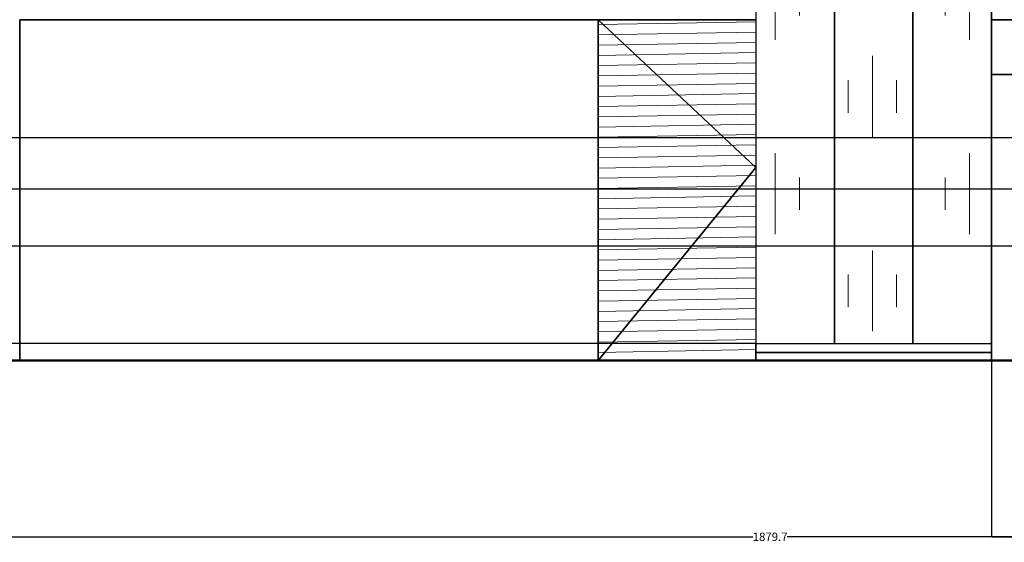
# Model space of a CAD drawing. Units: inches. Extents: x -1308 to 780, y 304 to 1023.
# Tile 3 of 7: x -667 to -138, y 304 to 585. Entities that reach past the tile are written whole.
import ezdxf

# ---------------------------------------------------------------- set-up
doc = ezdxf.new("R2010")
doc.units = ezdxf.units.IN
doc.header["$MEASUREMENT"] = 0
for name, color, linetype, lineweight in [('A-ANNO-DIMS', 2, 'Continuous', 18), ('A-ELEV', 7, 'Continuous', 35), ('A-ELEV-GRND', 7, 'Continuous', 50), ('A-ELEV-PATT', 8, 'Continuous', 13), ('A-GLAZ', 4, 'Continuous', 25)]:
    doc.layers.add(name, color=color, linetype=linetype, lineweight=lineweight)
doc.styles.get("Standard").update_dxf_attribs({"font": 'arial.ttf'})
doc.dimstyles.get("Standard").update_dxf_attribs({"dimtxt": 4.5, "dimasz": 0.18, "dimexe": 0.18, "dimexo": 0.0625, "dimgap": 0.09, "dimtad": 0, "dimtih": 1, "dimtoh": 1, "dimdec": 4, "dimzin": 0, "dimdsep": 46, "dimlunit": 4, "dimtxsty": 'Standard', "dimcen": 0.09, "dimadec": 0, "dimazin": 0, "dimtfac": 1, "dimtdec": 4, "dimtofl": 0, "dimtmove": 0, "dimatfit": 3, "dimfxl": 1, "dimtolj": 1, "dimtzin": 0, "dimarcsym": 0})

# ---------------------------------------------------------------- blocks, each defined once
blk = doc.blocks.new('*D1')
at = {"layer": 'A-ANNO-DIMS', "color": 0, "lineweight": -2, "transparency": 16777216}
for p, q in [((-1203.52, 401.95), (-1203.52, 307.09)), ((676.16, 401.95), (676.16, 307.09)), ((-1203.34, 307.27), (-272.9, 307.27)), ((675.98, 307.27), (-254.46, 307.27))]:
    blk.add_line(p, q, dxfattribs=at)
at = {"layer": 'A-ANNO-DIMS', "color": 0, "transparency": 16777216}
for points in [[(-1203.34, 307.3), (-1203.34, 307.24), (-1203.52, 307.27)], [(675.98, 307.3), (675.98, 307.24), (676.16, 307.27)]]:
    blk.add_solid(points, dxfattribs=at)
at = {"layer": 'Defpoints', "color": 0, "transparency": 16777216}
for p in [(-1203.52, 402.02), (676.16, 402.02), (676.16, 307.27)]:
    blk.add_point(p, dxfattribs=at)
at = {"layer": 'A-ANNO-DIMS', "color": 0, "transparency": 16777216, "insert": (-263.68, 307.27), "char_height": 4.5, "attachment_point": 5}
blk.add_mtext('\\A1;1879.7', dxfattribs=at)
blk = doc.blocks.new('*D9')
at = {"layer": 'A-ANNO-DIMS', "color": 0, "lineweight": -2, "transparency": 16777216}
for p, q in [((-144.73, 555.46), (-144.73, 307.09)), ((-129.95, 555.46), (-129.95, 307.09)), ((-144.55, 307.27), (-130.13, 307.27)), ((-129.95, 307.27), (-129.77, 307.27))]:
    blk.add_line(p, q, dxfattribs=at)
at = {"layer": 'A-ANNO-DIMS', "color": 0, "transparency": 16777216}
for points in [[(-144.55, 307.3), (-144.55, 307.24), (-144.73, 307.27)], [(-130.13, 307.3), (-130.13, 307.24), (-129.95, 307.27)]]:
    blk.add_solid(points, dxfattribs=at)
at = {"layer": 'Defpoints', "color": 0, "transparency": 16777216}
for p in [(-144.73, 555.52), (-129.95, 555.52), (-129.95, 307.27)]:
    blk.add_point(p, dxfattribs=at)
at = {"layer": 'A-ANNO-DIMS', "color": 0, "transparency": 16777216, "insert": (-120.55, 307.27), "char_height": 4.5, "attachment_point": 5}
blk.add_mtext('\\A1;14.787', dxfattribs=at)
blk = doc.blocks.new('*D45')
at = {"layer": 'A-ANNO-DIMS', "color": 0, "lineweight": -2, "transparency": 16777216}
for p, q in [((-25.86, 614.44), (-25.86, 307.09)), ((-144.73, 584.98), (-144.73, 307.09)), ((-144.55, 307.27), (-94.52, 307.27)), ((-26.04, 307.27), (-76.07, 307.27))]:
    blk.add_line(p, q, dxfattribs=at)
at = {"layer": 'A-ANNO-DIMS', "color": 0, "transparency": 16777216}
for points in [[(-144.55, 307.3), (-144.55, 307.24), (-144.73, 307.27)], [(-26.04, 307.3), (-26.04, 307.24), (-25.86, 307.27)]]:
    blk.add_solid(points, dxfattribs=at)
at = {"layer": 'Defpoints', "color": 0, "transparency": 16777216}
for p in [(-25.86, 614.51), (-144.73, 585.04), (-25.86, 307.27)]:
    blk.add_point(p, dxfattribs=at)
at = {"layer": 'A-ANNO-DIMS', "color": 0, "transparency": 16777216, "insert": (-85.3, 307.27), "char_height": 4.5, "attachment_point": 5}
blk.add_mtext('\\A1;118.88', dxfattribs=at)
blk = doc.blocks.new('*D57')
at = {"layer": 'A-ANNO-DIMS', "color": 0, "lineweight": -2, "transparency": 16777216}
for p, q in [((-628.74, 924.84), (-1298.45, 924.84)), ((-1298.27, 924.66), (-1298.27, 665.82)), ((-1298.27, 402.2), (-1298.27, 661.04)), ((-1203.58, 402.02), (-1298.45, 402.02))]:
    blk.add_line(p, q, dxfattribs=at)
at = {"layer": 'A-ANNO-DIMS', "color": 0, "transparency": 16777216}
for points in [[(-1298.3, 924.66), (-1298.24, 924.66), (-1298.27, 924.84)], [(-1298.3, 402.2), (-1298.24, 402.2), (-1298.27, 402.02)]]:
    blk.add_solid(points, dxfattribs=at)
at = {"layer": 'Defpoints', "color": 0, "transparency": 16777216}
for p in [(-1298.27, 924.84), (-628.68, 924.84), (-1203.52, 402.02)]:
    blk.add_point(p, dxfattribs=at)
at = {"layer": 'A-ANNO-DIMS', "color": 0, "transparency": 16777216, "insert": (-1298.27, 663.43), "char_height": 4.5, "attachment_point": 5}
blk.add_mtext('\\A1;522.8', dxfattribs=at)
blk = doc.blocks.new('*D58')
at = {"layer": 'A-ANNO-DIMS', "color": 0, "lineweight": -2, "transparency": 16777216}
for p, q in [((-1187.44, 521.84), (771.09, 521.84)), ((770.91, 521.66), (770.91, 464.32)), ((770.91, 402.2), (770.91, 459.54)), ((-1187.44, 402.02), (771.09, 402.02))]:
    blk.add_line(p, q, dxfattribs=at)
at = {"layer": 'A-ANNO-DIMS', "color": 0, "transparency": 16777216}
for points in [[(770.88, 521.66), (770.94, 521.66), (770.91, 521.84)], [(770.88, 402.2), (770.94, 402.2), (770.91, 402.02)]]:
    blk.add_solid(points, dxfattribs=at)
at = {"layer": 'Defpoints', "color": 0, "transparency": 16777216}
for p in [(-1187.5, 521.84), (770.91, 521.84), (-1187.5, 402.02)]:
    blk.add_point(p, dxfattribs=at)
at = {"layer": 'A-ANNO-DIMS', "color": 0, "transparency": 16777216, "insert": (770.91, 461.93), "char_height": 4.5, "attachment_point": 5}
blk.add_mtext('\\A1;119.83', dxfattribs=at)
blk = doc.blocks.new('*D63')
at = {"layer": 'A-ANNO-DIMS', "color": 0, "lineweight": -2, "transparency": 16777216}
for p, q in [((-843.54, 629.44), (771.09, 629.44)), ((770.91, 629.26), (770.91, 518.12)), ((770.91, 402.2), (770.91, 513.34)), ((-843.54, 402.02), (771.09, 402.02))]:
    blk.add_line(p, q, dxfattribs=at)
at = {"layer": 'A-ANNO-DIMS', "color": 0, "transparency": 16777216}
for points in [[(770.88, 629.26), (770.94, 629.26), (770.91, 629.44)], [(770.88, 402.2), (770.94, 402.2), (770.91, 402.02)]]:
    blk.add_solid(points, dxfattribs=at)
at = {"layer": 'Defpoints', "color": 0, "transparency": 16777216}
for p in [(-843.6, 629.44), (770.91, 629.44), (-843.6, 402.02)]:
    blk.add_point(p, dxfattribs=at)
at = {"layer": 'A-ANNO-DIMS', "color": 0, "transparency": 16777216, "insert": (770.91, 515.73), "char_height": 4.5, "attachment_point": 5}
blk.add_mtext('\\A1;227.43', dxfattribs=at)
blk = doc.blocks.new('*D67')
at = {"layer": 'A-ANNO-DIMS', "color": 0, "lineweight": -2, "transparency": 16777216}
for p, q in [((-271.41, 600.04), (-1298.45, 600.04)), ((-1298.27, 599.86), (-1298.27, 507.96)), ((-1298.27, 411.28), (-1298.27, 503.18)), ((-271.41, 411.1), (-1298.45, 411.1))]:
    blk.add_line(p, q, dxfattribs=at)
at = {"layer": 'A-ANNO-DIMS', "color": 0, "transparency": 16777216}
for points in [[(-1298.3, 599.86), (-1298.24, 599.86), (-1298.27, 600.04)], [(-1298.3, 411.28), (-1298.24, 411.28), (-1298.27, 411.1)]]:
    blk.add_solid(points, dxfattribs=at)
at = {"layer": 'Defpoints', "color": 0, "transparency": 16777216}
for p in [(-1298.27, 600.04), (-271.35, 600.04), (-271.35, 411.1)]:
    blk.add_point(p, dxfattribs=at)
at = {"layer": 'A-ANNO-DIMS', "color": 0, "transparency": 16777216, "insert": (-1298.27, 505.57), "char_height": 4.5, "attachment_point": 5}
blk.add_mtext('\\A1;188.94', dxfattribs=at)
blk = doc.blocks.new('*D79')
at = {"layer": 'A-ANNO-DIMS', "color": 0, "lineweight": -2, "transparency": 16777216}
for p, q in [((310.7, 463.43), (-1298.45, 463.43)), ((-1298.27, 463.25), (-1298.27, 435.11)), ((-1298.27, 402.2), (-1298.27, 430.34)), ((296.47, 402.02), (-1298.45, 402.02))]:
    blk.add_line(p, q, dxfattribs=at)
at = {"layer": 'A-ANNO-DIMS', "color": 0, "transparency": 16777216}
for points in [[(-1298.3, 463.25), (-1298.24, 463.25), (-1298.27, 463.43)], [(-1298.3, 402.2), (-1298.24, 402.2), (-1298.27, 402.02)]]:
    blk.add_solid(points, dxfattribs=at)
at = {"layer": 'Defpoints', "color": 0, "transparency": 16777216}
for p in [(-1298.27, 463.43), (310.77, 463.43), (296.53, 402.02)]:
    blk.add_point(p, dxfattribs=at)
at = {"layer": 'A-ANNO-DIMS', "color": 0, "transparency": 16777216, "insert": (-1298.27, 432.72), "char_height": 4.5, "attachment_point": 5}
blk.add_mtext('\\A1;61.42', dxfattribs=at)
blk = doc.blocks.new('*D80')
at = {"layer": 'A-ANNO-DIMS', "color": 0, "lineweight": -2, "transparency": 16777216}
for p, q in [((308.7, 494.07), (-1298.45, 494.07)), ((-1298.27, 493.89), (-1298.27, 481.14)), ((-1298.27, 463.61), (-1298.27, 476.36)), ((310.7, 463.43), (-1298.45, 463.43))]:
    blk.add_line(p, q, dxfattribs=at)
at = {"layer": 'A-ANNO-DIMS', "color": 0, "transparency": 16777216}
for points in [[(-1298.3, 493.89), (-1298.24, 493.89), (-1298.27, 494.07)], [(-1298.3, 463.61), (-1298.24, 463.61), (-1298.27, 463.43)]]:
    blk.add_solid(points, dxfattribs=at)
at = {"layer": 'Defpoints', "color": 0, "transparency": 16777216}
for p in [(-1298.27, 494.07), (308.77, 494.07), (310.77, 463.43)]:
    blk.add_point(p, dxfattribs=at)
at = {"layer": 'A-ANNO-DIMS', "color": 0, "transparency": 16777216, "insert": (-1298.27, 478.75), "char_height": 4.5, "attachment_point": 5}
blk.add_mtext('\\A1;30.64', dxfattribs=at)

msp = doc.modelspace()

# ---------------------------------------------------------------- hatches: boundary and pattern name
at = {"layer": 'A-ELEV-PATT'}
h = msp.add_hatch(dxfattribs=at)
h.set_pattern_fill('GOST_GLASS', color=256, scale=8.7, angle=45)
h.set_pattern_definition([(90, (0, 0), (52.2, 52.2), [43.5, -60.9]), (90, (13.05, 13.05), (52.2, 52.2), [17.4, -87]), (90, (-13.05, 13.05), (52.2, 52.2), [17.4, -87])])
h.paths.add_polyline_path([(-570.795, 854.0948), (-613.9558, 854.0948), (-613.9558, 755.0385), (-570.795, 755.0385)])
h.paths.add_polyline_path([(-499.4748, 854.0948), (-568.795, 854.0948), (-568.795, 755.0385), (-499.4748, 755.0385)])
h.paths.add_polyline_path([(-379.8352, 854.0948), (-497.4748, 854.0948), (-497.4748, 755.0385), (-379.8352, 755.0385)])
h.paths.add_polyline_path([(-292.4461, 854.0948), (-377.8352, 854.0948), (-377.8352, 755.0385), (-292.4461, 755.0385)])
h.paths.add_polyline_path([(4.0783, 875.1709), (-63.0069, 875.1709), (-63.0069, 753.0385), (4.0783, 753.0385)])
h.paths.add_polyline_path([(77.4055, 875.1709), (6.0783, 875.1709), (6.0783, 753.0385), (77.4055, 753.0385)])
h.paths.add_polyline_path([(150.9148, 814.1047), (79.4055, 814.1047), (79.4055, 753.0385), (150.9148, 753.0385)])
h.paths.add_polyline_path([(110.9181, 875.1709), (79.4055, 875.1709), (79.4055, 814.1047)])
h.paths.add_polyline_path([(150.9148, 875.1709), (110.9181, 875.1709), (149.6048, 816.1047), (150.9148, 816.1047)])
h.paths.add_polyline_path([(-227.6882, 875.1709), (-271.346, 875.1709), (-271.346, 753.0385), (-227.6882, 753.0385)])
h.paths.add_polyline_path([(-188.3907, 875.1709), (-227.6882, 875.1709), (-227.6882, 753.0385), (-188.3907, 753.0385)])
h.paths.add_polyline_path([(-144.7329, 875.1709), (-188.3907, 875.1709), (-188.3907, 753.0385), (-144.7329, 753.0385)])
h.paths.add_polyline_path([(-144.7329, 739.0259), (-188.3907, 739.0259), (-188.3907, 624.4429), (-144.7329, 624.4429)])
h.paths.add_polyline_path([(-188.3907, 739.0259), (-227.6882, 739.0259), (-227.6882, 624.4429), (-188.3907, 624.4429)])
h.paths.add_polyline_path([(-227.6882, 739.0259), (-271.346, 739.0259), (-271.346, 624.4429), (-227.6882, 624.4429)])
h.paths.add_polyline_path([(-229.1416, 600.0434), (-271.346, 600.0434), (-271.346, 411.1006), (-229.1416, 411.1006)])
h.paths.add_polyline_path([(-186.9373, 600.0434), (-229.1416, 600.0434), (-229.1416, 411.1006), (-186.9373, 411.1006)])
h.paths.add_polyline_path([(-144.7329, 600.0434), (-186.9373, 600.0434), (-186.9373, 411.1006), (-144.7329, 411.1006)])
h = msp.add_hatch(dxfattribs=at)
h.set_pattern_fill('ANSI31', color=256, scale=44, angle=136)
h.paths.add_polyline_path([(-271.346, 505.572), (-356.0562, 585.0385), (-356.0562, 402.0158)])
h.paths.add_polyline_path([(-271.346, 585.0385), (-356.0562, 585.0385), (-271.346, 505.572)], flags=17)
h.paths.add_polyline_path([(-271.346, 505.572), (-356.0562, 402.0158), (-271.346, 402.0158), (-271.346, 406.2371), (-271.346, 411.1006)], flags=17)

# ---------------------------------------------------------------- linework, layer by layer
at = {"layer": 'A-ELEV'}
for p, q in [((-144.7329, 753.0385), (-144.7329, 585.0385)), ((-666.946, 402.0158), (-666.946, 585.0385)), ((-666.946, 585.0385), (-557.1914, 585.0385)), ((-271.346, 585.0385), (-557.1914, 585.0385)), ((-356.0562, 585.0385), (-356.0562, 402.0158)), ((-356.0562, 585.0385), (-271.346, 505.572)), ((-144.7329, 555.5236), (-144.7329, 585.0385)), ((-144.7329, 585.0385), (526.9606, 585.0385)), ((50.6624, 555.5236), (-144.7329, 555.5236)), ((-144.7329, 555.5236), (-144.7329, 402.0158)), ((-271.346, 505.572), (-356.0562, 402.0158)), ((-271.346, 411.1006), (-271.346, 406.2371)), ((-271.346, 406.2371), (-144.7329, 406.2371)), ((-271.346, 406.2371), (-271.346, 402.0158))]:
    msp.add_line(p, q, dxfattribs=at)
at = {"layer": 'A-ELEV-GRND'}
for p, q in [((-608.7933, 402.0158), (-725.0987, 402.0158)), ((-144.7329, 402.0158), (-608.7933, 402.0158)), ((47.1224, 402.0158), (-144.7329, 402.0158))]:
    msp.add_line(p, q, dxfattribs=at)
at = {"layer": 'A-GLAZ'}
for points in [[(-229.1416, 600.0434), (-271.346, 600.0434), (-271.346, 411.1006), (-229.1416, 411.1006)], [(-186.9373, 600.0434), (-229.1416, 600.0434), (-229.1416, 411.1006), (-186.9373, 411.1006)], [(-144.7329, 600.0434), (-186.9373, 600.0434), (-186.9373, 411.1006), (-144.7329, 411.1006)]]:
    msp.add_lwpolyline(points, close=True, dxfattribs=at)

# ---------------------------------------------------------------- dimensions: what is measured, and where the dimension line sits
at = {"layer": 'A-ANNO-DIMS'}
for base, p1, p2, override, picture, middle in [((-1298.268, 924.8421), (-1203.518, 402.0158), (-628.6809, 924.8421), {"dimdec": 1, "dimlfac": 1, "dimrnd": 0, "dimzin": 0, "dimdsep": 46, "dimlunit": 2}, '*D57', (-1298.268, 663.429)), ((770.9076, 629.4421), (-843.5988, 402.0158), (-843.5988, 629.4421), {"dimdec": 2, "dimlfac": 1, "dimrnd": 0, "dimzin": 0, "dimdsep": 46, "dimlunit": 2}, '*D63', (770.9076, 515.729)), ((-1298.268, 600.0434), (-271.346, 411.1006), (-271.346, 600.0434), {"dimdec": 2, "dimlfac": 1, "dimrnd": 0, "dimzin": 0, "dimdsep": 46, "dimlunit": 2}, '*D67', (-1298.268, 505.572)), ((770.9076, 521.8442), (-1187.498, 402.0158), (-1187.498, 521.8442), {"dimdec": 2, "dimlfac": 1, "dimrnd": 0, "dimzin": 0, "dimdsep": 46, "dimlunit": 2}, '*D58', (770.9076, 461.93)), ((-1298.268, 494.0703), (310.7651, 463.4331), (308.7651, 494.0703), {"dimdec": 2, "dimlfac": 1, "dimrnd": 0, "dimzin": 0, "dimdsep": 46, "dimlunit": 2}, '*D80', (-1298.268, 478.7517)), ((-1298.268, 463.4331), (296.5309, 402.0158), (310.7651, 463.4331), {"dimdec": 2, "dimlfac": 1, "dimrnd": 0, "dimzin": 0, "dimdsep": 46, "dimlunit": 2}, '*D79', (-1298.268, 432.7245))]:
    dim = msp.add_linear_dim(base=base, p1=p1, p2=p2, angle=90, dimstyle='Standard', override=override, dxfattribs=at)
    dim.commit()
    dim.dimension.update_dxf_attribs({"geometry": picture, "text_midpoint": middle})
for base, p1, p2, override, picture, middle in [((-25.8575, 307.2658), (-144.7329, 585.0385), (-25.8575, 614.5069), {"dimdec": 2, "dimlfac": 1, "dimrnd": 0, "dimzin": 0, "dimdsep": 46, "dimlunit": 2}, '*D45', (-85.2952, 307.2658)), ((-129.9455, 307.2658), (-144.7329, 555.5236), (-129.9455, 555.5236), {"dimdec": 3, "dimlfac": 1, "dimrnd": 0, "dimzin": 0, "dimdsep": 46, "dimlunit": 2}, '*D9', (-120.5466, 307.2658)), ((676.1576, 307.2658), (-1203.518, 402.0158), (676.1576, 402.0158), {"dimdec": 1, "dimlfac": 1, "dimrnd": 0, "dimzin": 0, "dimdsep": 46, "dimlunit": 2}, '*D1', (-263.6802, 307.2658))]:
    dim = msp.add_linear_dim(base=base, p1=p1, p2=p2, dimstyle='Standard', override=override, dxfattribs=at)
    dim.commit()
    dim.dimension.update_dxf_attribs({"geometry": picture, "text_midpoint": middle})

doc.saveas('drawing.dxf')
